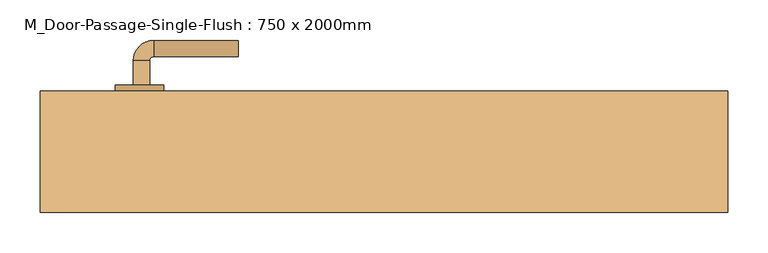
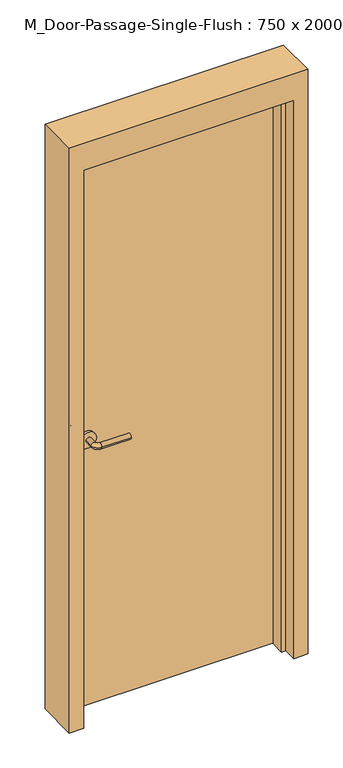
"""IFC4 building model written with IfcOpenShell, lengths in millimetres: door geometry, M_Door-Passage-Single-Flush : 750 x 2000mm."""

from ifc_helpers import new_model, si_unit, point, frame, frame_2d, origin, origin_with_axes, place, context, project, spatial, polyline, circle_curve, ellipse_curve, trimmed, segment, composite_curve, outline, extrude, faceted_brep, source, transform, mapped, element, save
from ifc_brep_helpers import plane_surface, cylinder_surface, revolved_surface, advanced_brep


def m_door_passage_single_flush_750_x_2000mm_a9826c90(model_context):
    return source(origin(), model_context, "Body", "SolidModel", [
        advanced_brep(
        [(-309.990625, 3.35, 1000.0), (-289.990625, 3.35, 1000.0), (-289.990625, -26.65, 1000.0), (-309.990625, -26.65, 1000.0), (-284.990625, -31.65, 1000.0), (-284.990625, -51.65, 1000.0), (-179.990625, -51.65, 1000.0), (-179.990625, -31.65, 1000.0)],
        [
            (0, 1, circle_curve(frame((-299.990625, 3.35, 1000.0), z_axis=(0.0, 1.0, 0.0), x_axis=(1.0, 0.0, 0.0)), 10.0)),
            (1, 0, circle_curve(frame((-299.990625, 3.35, 1000.0), z_axis=(0.0, 1.0, 0.0), x_axis=(1.0, 0.0, 0.0)), 10.0)),
            (1, 2),
            (2, 3, circle_curve(frame((-299.990625, -26.65, 1000.0), z_axis=(0.0, 1.0, 0.0), x_axis=(1.0, 0.0, 0.0)), 10.0)),
            (3, 0),
            (3, 2, circle_curve(frame((-299.990625, -26.65, 1000.0), z_axis=(0.0, 1.0, 0.0), x_axis=(1.0, 0.0, 0.0)), 10.0)),
            (4, 5, circle_curve(frame((-284.990625, -41.65, 1000.0), z_axis=(-1.0, 0.0, 0.0), x_axis=(0.0, 1.0, 0.0)), 10.0)),
            (5, 3, circle_curve(frame((-284.990625, -26.65, 1000.0), z_axis=(0.0, 0.0, -1.0), x_axis=(-1.0, 0.0, 0.0)), 25.0)),
            (2, 4, circle_curve(frame((-284.990625, -26.65, 1000.0), z_axis=(0.0, 0.0, 1.0), x_axis=(-1.0, 0.0, 0.0)), 5.0)),
            (5, 4, circle_curve(frame((-284.990625, -41.65, 1000.0), z_axis=(-1.0, 0.0, 0.0), x_axis=(0.0, 1.0, 0.0)), 10.0)),
            (6, 7, circle_curve(frame((-179.990625, -41.65, 1000.0), z_axis=(1.0, 0.0, 0.0), x_axis=(0.0, 1.0, 0.0)), 10.0)),
            (7, 6, circle_curve(frame((-179.990625, -41.65, 1000.0), z_axis=(1.0, 0.0, 0.0), x_axis=(0.0, 1.0, 0.0)), 10.0)),
            (4, 7),
            (6, 5),
        ],
        [
            plane_surface(frame((-299.990625, 3.35, 1000.0), z_axis=(0.0, 1.0, 0.0), x_axis=(0.0, 0.0, 1.0))),
            cylinder_surface(frame((-299.990625, 3.35, 1000.0), z_axis=(0.0, 1.0, 0.0), x_axis=(1.0, 0.0, 0.0)), 10.0),
            revolved_surface(trimmed(ellipse_curve(frame((-299.990625, -26.65, 1000.0), z_axis=(0.0, -1.0, 0.0), x_axis=(1.0, 0.0, 0.0)), 10.0, 10.0), [point((-309.990625, -26.65, 1000.0))], [point((-289.990625, -26.65, 1000.0))], True, "CARTESIAN"), (-284.990625, -26.65, 1000.0), (0.0, 0.0, -1.0)),
            revolved_surface(trimmed(ellipse_curve(frame((-299.990625, -26.65, 1000.0), z_axis=(0.0, -1.0, 0.0), x_axis=(1.0, 0.0, 0.0)), 10.0, 10.0), [point((-289.990625, -26.65, 1000.0))], [point((-309.990625, -26.65, 1000.0))], True, "CARTESIAN"), (-284.990625, -26.65, 1000.0), (0.0, 0.0, -1.0)),
            plane_surface(frame((-179.990625, -41.65, 1000.0), z_axis=(1.0, 0.0, 0.0), x_axis=(0.0, 0.0, 1.0))),
            cylinder_surface(frame((-284.990625, -41.65, 1000.0), z_axis=(-1.0, 0.0, 0.0), x_axis=(0.0, 1.0, 0.0)), 10.0),
        ],
        [
            (0, [[1, 2]]),
            (1, [[3, 4, 5, -2]]),
            (1, [[-5, 6, -3, -1]]),
            (2, [[7, 8, -4, 9]]),
            (3, [[10, -9, -6, -8]]),
            (4, [[11, 12]]),
            (5, [[13, -11, 14, -7]]),
            (5, [[-14, -12, -13, -10]]),
        ],
    ),
        extrude(outline(composite_curve([segment(trimmed(circle_curve(frame_2d((1000.0, -302.490625)), 30.0), [point((1000.0, -332.490625))], [point((1000.0, -272.490625))], False, "CARTESIAN"), True, "CONTINUOUS"), segment(trimmed(circle_curve(frame_2d((1000.0, -302.490625)), 30.0), [point((1000.0, -272.490625))], [point((1000.0, -332.490625))], False, "CARTESIAN"), True, "CONTINUOUS")], self_intersect=False)), frame((0.0, 3.35, 0.0), z_axis=(0.0, 1.0, 0.0), x_axis=(0.0, 0.0, 1.0)), (0.0, 0.0, 1.0), 8.0),
        advanced_brep(
        [(-309.990625, 64.35, 1000.0), (-289.990625, 64.35, 1000.0), (-309.990625, 94.35, 1000.0), (-289.990625, 94.35, 1000.0), (-284.990625, 99.35, 1000.0), (-284.990625, 119.35, 1000.0), (-179.990625, 119.35, 1000.0), (-179.990625, 99.35, 1000.0)],
        [
            (0, 1, circle_curve(frame((-299.990625, 64.35, 1000.0), z_axis=(0.0, -1.0, 0.0), x_axis=(1.0, 0.0, 0.0)), 10.0)),
            (1, 0, circle_curve(frame((-299.990625, 64.35, 1000.0), z_axis=(0.0, -1.0, 0.0), x_axis=(1.0, 0.0, 0.0)), 10.0)),
            (0, 2),
            (2, 3, circle_curve(frame((-299.990625, 94.35, 1000.0), z_axis=(0.0, -1.0, 0.0), x_axis=(1.0, 0.0, 0.0)), 10.0)),
            (3, 1),
            (3, 2, circle_curve(frame((-299.990625, 94.35, 1000.0), z_axis=(0.0, -1.0, 0.0), x_axis=(1.0, 0.0, 0.0)), 10.0)),
            (4, 3, circle_curve(frame((-284.990625, 94.35, 1000.0), z_axis=(0.0, 0.0, 1.0), x_axis=(-1.0, 0.0, 0.0)), 5.0)),
            (2, 5, circle_curve(frame((-284.990625, 94.35, 1000.0), z_axis=(0.0, 0.0, -1.0), x_axis=(-1.0, 0.0, 0.0)), 25.0)),
            (5, 4, circle_curve(frame((-284.990625, 109.35, 1000.0), z_axis=(-1.0, 0.0, 0.0), x_axis=(0.0, -1.0, 0.0)), 10.0)),
            (4, 5, circle_curve(frame((-284.990625, 109.35, 1000.0), z_axis=(-1.0, 0.0, 0.0), x_axis=(0.0, -1.0, 0.0)), 10.0)),
            (6, 7, circle_curve(frame((-179.990625, 109.35, 1000.0), z_axis=(1.0, 0.0, 0.0), x_axis=(0.0, -1.0, 0.0)), 10.0)),
            (7, 6, circle_curve(frame((-179.990625, 109.35, 1000.0), z_axis=(1.0, 0.0, 0.0), x_axis=(0.0, -1.0, 0.0)), 10.0)),
            (5, 6),
            (7, 4),
        ],
        [
            plane_surface(frame((-299.990625, 64.35, 1000.0), z_axis=(0.0, -1.0, 0.0), x_axis=(0.0, 0.0, 1.0))),
            cylinder_surface(frame((-299.990625, 64.35, 1000.0), z_axis=(0.0, -1.0, 0.0), x_axis=(1.0, 0.0, 0.0)), 10.0),
            revolved_surface(trimmed(ellipse_curve(frame((-299.990625, 94.35, 1000.0), z_axis=(0.0, -1.0, 0.0), x_axis=(1.0, 0.0, 0.0)), 10.0, 10.0), [point((-309.990625, 94.35, 1000.0))], [point((-289.990625, 94.35, 1000.0))], True, "CARTESIAN"), (-284.990625, 94.35, 1000.0), (0.0, 0.0, -1.0)),
            revolved_surface(trimmed(ellipse_curve(frame((-299.990625, 94.35, 1000.0), z_axis=(0.0, -1.0, 0.0), x_axis=(1.0, 0.0, 0.0)), 10.0, 10.0), [point((-289.990625, 94.35, 1000.0))], [point((-309.990625, 94.35, 1000.0))], True, "CARTESIAN"), (-284.990625, 94.35, 1000.0), (0.0, 0.0, -1.0)),
            plane_surface(frame((-179.990625, 109.35, 1000.0), z_axis=(1.0, 0.0, 0.0), x_axis=(0.0, 0.0, 1.0))),
            cylinder_surface(frame((-284.990625, 109.35, 1000.0), z_axis=(-1.0, 0.0, 0.0), x_axis=(0.0, -1.0, 0.0)), 10.0),
        ],
        [
            (0, [[1, 2]]),
            (1, [[-1, 3, 4, 5]]),
            (1, [[-2, -5, 6, -3]]),
            (2, [[7, -4, 8, 9]]),
            (3, [[-8, -6, -7, 10]]),
            (4, [[11, 12]]),
            (5, [[-9, 13, -12, 14]]),
            (5, [[-10, -14, -11, -13]]),
        ],
    ),
        extrude(outline(composite_curve([segment(trimmed(circle_curve(frame_2d((1000.0, -302.490625)), 30.0), [point((1000.0, -332.490625))], [point((1000.0, -272.490625))], False, "CARTESIAN"), True, "CONTINUOUS"), segment(trimmed(circle_curve(frame_2d((1000.0, -302.490625)), 30.0), [point((1000.0, -272.490625))], [point((1000.0, -332.490625))], False, "CARTESIAN"), True, "CONTINUOUS")], self_intersect=False)), frame((0.0, 56.35, 0.0), z_axis=(0.0, 1.0, 0.0), x_axis=(0.0, 0.0, 1.0)), (0.0, 0.0, 1.0), 8.0),
        extrude(outline(polyline([(375.0, 11.35), (-375.0, 11.35), (-375.0, 56.35), (375.0, 56.35), (375.0, 11.35)])), origin_with_axes(), (0.0, 0.0, 1.0), 2100.0),
        faceted_brep([(375.0, 6.5875, 0.0), (375.0, 56.35, 0.0), (425.0, 56.35, 0.0), (425.0, -93.65, 0.0), (375.0, -93.65, 0.0), (375.0, -44.4375, 0.0), (359.125, -44.4375, 0.0), (359.125, 6.5875, 0.0), (375.0, 6.5875, 2100.0), (375.0, 56.35, 2100.0), (-375.0, 56.35, 2100.0), (-375.0, 56.35, 0.0), (-425.0, 56.35, 0.0), (-425.0, 56.35, 2200.0), (425.0, 56.35, 2200.0), (425.0, -93.65, 2200.0), (-425.0, -93.65, 2200.0), (-425.0, -93.65, 0.0), (-375.0, -93.65, 0.0), (-375.0, -93.65, 2100.0), (375.0, -93.65, 2100.0), (375.0, -44.4375, 2100.0), (-375.0, -44.4375, 2100.0), (-375.0, -44.4375, 0.0), (-359.125, -44.4375, 0.0), (-359.125, -44.4375, 2084.125), (359.125, -44.4375, 2084.125), (359.125, 6.5875, 2084.125), (-359.125, 6.5875, 2084.125), (-359.125, 6.5875, 0.0), (-375.0, 6.5875, 0.0), (-375.0, 6.5875, 2100.0)], [[[0, 1, 2, 3, 4, 5, 6, 7]], [[1, 0, 8, 9]], [[2, 1, 9, 10, 11, 12, 13, 14]], [[3, 2, 14, 15]], [[4, 3, 15, 16, 17, 18, 19, 20]], [[5, 4, 20, 21]], [[6, 5, 21, 22, 23, 24, 25, 26]], [[7, 6, 26, 27]], [[0, 7, 27, 28, 29, 30, 31, 8]], [[9, 8, 31, 10]], [[20, 19, 22, 21]], [[26, 25, 28, 27]], [[12, 11, 30, 29, 24, 23, 18, 17]], [[11, 10, 31, 30]], [[13, 12, 17, 16]], [[19, 18, 23, 22]], [[25, 24, 29, 28]], [[15, 14, 13, 16]]]),
    ])


if __name__ == "__main__":
    model = new_model("IFC4")
    model_context = context("Model", 3, world=origin())
    ifc_project = project(units=[si_unit("LENGTHUNIT", "METRE", prefix="MILLI")], contexts=[model_context])
    site = spatial("IfcSite", under=ifc_project)
    building = spatial("IfcBuilding", under=site)
    placement = place(None, origin())
    m_door_passage_single_flush_750_x_2000mm_shape = m_door_passage_single_flush_750_x_2000mm_a9826c90(model_context)
    element("IfcDoor", 1, ObjectType="M_Door-Passage-Single-Flush : 750 x 2000mm", at=placement, inside=building, context=model_context, shape_type="MappedRepresentation", body=[
        mapped(m_door_passage_single_flush_750_x_2000mm_shape, transform((0.0, 0.0, 0.0), x_axis=(1.0, 0.0, 0.0), y_axis=(0.0, 1.0, 0.0), z_axis=(0.0, 0.0, 1.0))),
    ])
    save(model, "model.ifc")

# Revit data of these elements
# Type "M_Door-Passage-Single-Flush : 750 x 2000mm"
#   Type Mark = "35"
#   Assembly Code = "B2030200"
#   Analytic Construction = "Wooden"
#   Thickness = 45 mm
#   Thermal Resistance (R) = 0.455703 (m²·K)/W
#   Swing Angle [instance default] = 90.00°
#   Strike Height = 1000 mm
#   Rough Width [instance default] = 850 mm
#   Rough Height [instance default] = 2200 mm
#   MF Opening Height [instance default] = 100 mm
#   MF Opening Width [instance default] = 100 mm
#   Inset Calculate [instance default] = 105 mm
#   Masonry Inset [instance default] = 25 mm
#   Height = 2100 mm
#   Width = 750 mm
#   Heat Transfer Coefficient (U) = 2.19465 W/(m²·K)
#   Masonry Frame Depth = 150 mm
#   Masonry Frame [instance default] = yes
#   Function = 1
#   Dry Wall Frame [instance default] = no
#   Panel Material = Wood - Birch
#   Frame Material = Metal - Paint Finish - Grey
#   Door Handle Material = Aluminum
#   Visual Light Transmittance = 0
#   Solar Heat Gain Coefficient = 0
#   Wall Closure = (empty or 0)
# Element 1 (IfcDoor, "M_Door-Passage-Single-Flush : 750 x 2000mm")
#   Materials on its faces: "Aluminum", "Metal - Paint Finish - Grey", "Wood - Birch"
# Materials
#   "Wood - Birch": class "Wood", colour RGB 173 132 96, transparency 0, Cost = 0
#   "Metal - Paint Finish - Grey": class "Paint", colour RGB 178 178 178, transparency 0, Cost = 0
#   "Aluminum": class "Metal", colour RGB 244 245 246, transparency 0, Description = "Aluminum 6061", Cost = 0
